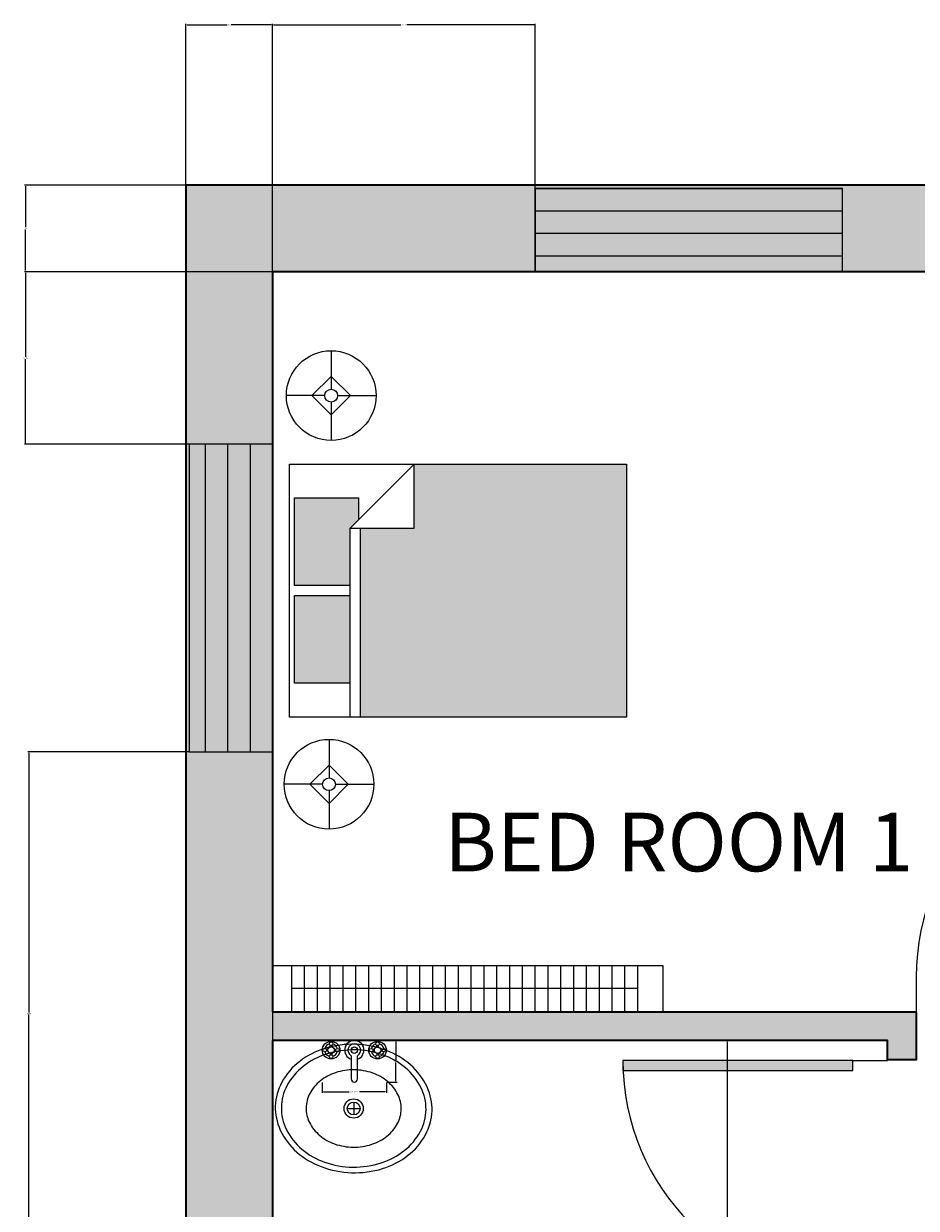
# Model space of a CAD drawing. Units: inches. Extents: x 1434 to 1845, y 1483 to 2014.
# Tile 9 of 11: x 1434 to 1573, y 1829 to 2014. Entities that reach past the tile are written whole.
import ezdxf

# ---------------------------------------------------------------- set-up
doc = ezdxf.new("R2010")
doc.units = ezdxf.units.IN
for name, color, linetype, lineweight in [('A-ANNO-DIMS', 2, 'Continuous', 18), ('A-AREA-IDEN', 7, 'Continuous', 25), ('A-DOOR', 3, 'Continuous', 25), ('A-FLOR-FIXT', 8, 'Continuous', 18), ('A-FLOR-FIXT-PATT', 8, 'Continuous', 13), ('A-FURN', 9, 'Continuous', 18), ('A-FURN-PATT', 9, 'Continuous', 13), ('A-GLAZ', 4, 'Continuous', 18), ('A-GLAZ-PATT', 9, 'Continuous', 13), ('A-WALL', 7, 'Continuous', 35), ('A-WALL-PATT', 8, 'Continuous', 13), ('E-LITE', 2, 'Continuous', 18)]:
    doc.layers.add(name, color=color, linetype=linetype, lineweight=lineweight)
doc.layers.add('A-DOOR-PATT', color=39, linetype='Continuous', lineweight=13, true_color=0x58382b)
doc.styles.get("Standard").update_dxf_attribs({"font": 'arial.ttf'})
doc.dimstyles.get("Standard").update_dxf_attribs({"dimtxt": 0.18, "dimasz": 0.18, "dimexe": 0.18, "dimexo": 0.0625, "dimgap": 0.09, "dimtad": 0, "dimtih": 1, "dimtoh": 1, "dimdec": 4, "dimzin": 0, "dimdsep": 46, "dimtxsty": 'Standard', "dimcen": 0.09, "dimadec": 0, "dimazin": 0, "dimtfac": 1, "dimtdec": 4, "dimtofl": 0, "dimtmove": 0, "dimatfit": 3, "dimfxl": 1, "dimtolj": 1, "dimtzin": 0, "dimarcsym": 0})

# ---------------------------------------------------------------- blocks, each defined once
blk = doc.blocks.new('*U2')
for p, q in [((0, 0), (0, -6)), ((-40, 0), (-40, -6))]:
    blk.add_line(p, q)
blk.add_lwpolyline([(0, 0), (0, 40), (-1.75, 40), (-1.75, 0)], close=True)
blk.add_arc((0, 0), 40, 90, 180)
blk = doc.blocks.new('Bed - Queen')
for p, q in [((0, -80.00003), (0, 0)), ((0, 0), (59.99999, 0)), ((59.99999, 0), (59.99999, -80.00003)), ((7.99999, -1.2), (28.79998, -1.2)), ((7.99999, -14.4), (7.99999, -1.2)), ((28.79998, -1.2), (28.79998, -14.4)), ((31.19999, -1.2), (51.99999, -1.2)), ((31.19999, -14.4), (31.19999, -1.2)), ((51.99999, -1.2), (51.99999, -16.4)), ((0, -14.4), (44.8, -14.4)), ((44.8, -16.8), (0, -16.8)), ((59.99999, -29.6), (44.8, -14.4)), ((44.8, -14.4), (44.8, -29.6)), ((51.99999, -16.4), (46.79936, -16.4)), ((44.8, -29.6), (59.99999, -29.6)), ((59.99999, -80.00003), (0, -80.00003))]:
    blk.add_line(p, q)
blk = doc.blocks.new('Lamp - Table')
for p, q in [((0, 7), (0, 1)), ((0, 3), (-3, 0)), ((3, 0), (0, 3)), ((-1, 0), (-7, 0)), ((-3, 0), (0, -3)), ((0, -3), (3, 0)), ((1, 0), (7, 0)), ((0, -1), (0, -7))]:
    blk.add_line(p, q)
for radius in [7, 1]:
    blk.add_circle((0, 0), radius)
blk = doc.blocks.new('Sink - Oval top')
for p, q in [((-1, 0), (1, 0)), ((0, 1), (0, -1))]:
    blk.add_line(p, q)
for points in [[(-12.23, 0.39, 0.117634), (-11.46, -3.36, 0.104469), (-8.88, -6.8, 0.090016), (-5.08, -9.07, 0.08192), (-0.32, -10.02, 0.08192), (4.49, -9.38, 0.090016), (8.42, -7.36, 0.104469), (11.22, -4.09, 0.117634), (12.23, -0.39, 0.117634), (11.46, 3.36, 0.104469), (8.88, 6.8, 0.090016), (5.08, 9.07, 0.08192), (0.32, 10.02, 0.08192), (-4.49, 9.38, 0.090016), (-8.42, 7.36, 0.104469), (-11.22, 4.09, 0.117634)], [(-11.29, 0.16, 0.118622), (-10.52, -3.25, 0.104678), (-8.07, -6.36, 0.089562), (-4.54, -8.37, 0.081185), (-0.13, -9.15, 0.081185), (4.3, -8.49, 0.089562), (7.89, -6.58, 0.104678), (10.42, -3.55, 0.118622), (11.29, -0.16, 0.118622), (10.52, 3.25, 0.104678), (8.07, 6.36, 0.089562), (4.54, 8.37, 0.081185), (0.13, 9.15, 0.081185), (-4.3, 8.49, 0.089562), (-7.89, 6.58, 0.104678), (-10.42, 3.55, 0.118622)], [(-7.42, 0.08, 0.118283), (-6.91, -2.17, 0.104607), (-5.29, -4.21, 0.089718), (-2.97, -5.53, 0.081436), (-0.07, -6.04, 0.081436), (2.84, -5.59, 0.089718), (5.2, -4.33, 0.104607), (6.86, -2.32, 0.118283), (7.42, -0.08, 0.118283), (6.91, 2.17, 0.104607), (5.29, 4.21, 0.089718), (2.97, 5.53, 0.081436), (0.07, 6.04, 0.081436), (-2.84, 5.59, 0.089718), (-5.2, 4.33, 0.104607), (-6.86, 2.32, 0.118283)]]:
    blk.add_lwpolyline(points, format="xyb", close=True)
for radius in [1.5, 1]:
    blk.add_circle((0, 0), radius)
blk = doc.blocks.new('Faucet - Bathroom top')
for p, q in [((-4.107, 0.125), (-4.375, 0.125)), ((-3.75, 0.4788), (-3.75, 0.75)), ((-3.5, 0.482), (-3.5, 0.75)), ((-3.1461, 0.125), (-2.875, 0.125)), ((3.143, 0.125), (2.875, 0.125)), ((3.5, 0.4788), (3.5, 0.75)), ((3.75, 0.482), (3.75, 0.75)), ((4.1039, 0.125), (4.375, 0.125)), ((-4.1039, -0.125), (-4.375, -0.125)), ((-3.75, -0.4821), (-3.75, -0.75)), ((-3.5, -0.4789), (-3.5, -0.75)), ((-3.143, -0.125), (-2.875, -0.125)), ((-0.5, -0.8639), (-0.5, -4.5)), ((0.5, -4.5), (0.5, -0.8631)), ((3.1461, -0.125), (2.875, -0.125)), ((3.5, -0.4821), (3.5, -0.75)), ((3.75, -0.4789), (3.75, -0.75)), ((4.107, -0.125), (4.375, -0.125))]:
    blk.add_line(p, q)
for centre, radius in [((-3.625, 0), 1.375), ((-4.625, 0), 0.2795), ((-3.625, 0), 0.5), ((-3.625, 1), 0.2795), ((-2.625, 0), 0.2795), ((0, 0), 0.5), ((3.625, 0), 1.375), ((2.625, 0), 0.2795), ((3.625, 0), 0.5), ((3.625, 1), 0.2795), ((4.625, 0), 0.2795), ((-3.625, -1), 0.2795), ((3.625, -1), 0.2795)]:
    blk.add_circle(centre, radius)
for centre, radius, start, end in [((-3.625, 0), 1, 105.2407, 164.2093), ((-3.625, 0), 1, 16.44125, 74.07887), ((0, 0), 1.5, 289.6514, 250.3603), ((0, 0), 1, 300.3431, 239.7554), ((3.625, 0), 1, 106.12, 164.0884), ((3.625, 0), 1, 16.23422, 73.90469), ((-3.625, 0), 1, 196.2342, 253.9047), ((-3.625, 0), 1, 286.12, 344.0884), ((3.625, 0), 1, 196.4413, 254.0789), ((3.625, 0), 1, 285.2407, 344.2093), ((0, -4.5), 0.5, 180, 0)]:
    blk.add_arc(centre, radius, start, end)
blk = doc.blocks.new('WIN-48IN-13IN')
for p, q in [((13, 48), (0, 48)), ((0, 48), (0, 12)), ((2.5, 48), (2.5, 0)), ((6, 48), (6, 0)), ((9.5, 48), (9.5, 0)), ((0, 12), (0, 0)), ((0, 0), (13, 0))]:
    blk.add_line(p, q)
blk.add_lwpolyline([(13, 48), (13, 0)], close=True)
blk = doc.blocks.new('*D34')
at = {"layer": 'A-ANNO-DIMS', "color": 0, "lineweight": -2, "transparency": 16777216}
for p, q in [((1480.75, 1848.31), (1480.75, 1846.69)), ((1480.93, 1846.87), (1484.94, 1846.87)), ((1490.57, 1846.87), (1486.56, 1846.87)), ((1490.75, 1848.31), (1490.75, 1846.69))]:
    blk.add_line(p, q, dxfattribs=at)
at = {"layer": 'A-ANNO-DIMS', "color": 0, "transparency": 16777216}
for points in [[(1480.93, 1846.9), (1480.93, 1846.84), (1480.75, 1846.87)], [(1490.57, 1846.9), (1490.57, 1846.84), (1490.75, 1846.87)]]:
    blk.add_solid(points, dxfattribs=at)
at = {"layer": 'Defpoints', "color": 0, "transparency": 16777216}
for p in [(1480.75, 1848.37), (1490.75, 1848.37), (1490.75, 1846.87)]:
    blk.add_point(p, dxfattribs=at)
at = {"layer": 'A-ANNO-DIMS', "color": 0, "transparency": 16777216, "insert": (1485.75, 1846.87), "char_height": 0.18, "attachment_point": 5}
blk.add_mtext('\\A1;TAP 10 TYP.', dxfattribs=at)
blk = doc.blocks.new('*D35')
at = {"layer": 'A-ANNO-DIMS', "color": 0, "lineweight": -2, "transparency": 16777216}
for p, q in [((1490.81, 1854.87), (1492.43, 1854.87)), ((1492.25, 1854.69), (1492.25, 1851.8)), ((1492.25, 1848.55), (1492.25, 1851.44)), ((1490.81, 1848.37), (1492.43, 1848.37))]:
    blk.add_line(p, q, dxfattribs=at)
at = {"layer": 'A-ANNO-DIMS', "color": 0, "transparency": 16777216}
for points in [[(1492.22, 1854.69), (1492.28, 1854.69), (1492.25, 1854.87)], [(1492.22, 1848.55), (1492.28, 1848.55), (1492.25, 1848.37)]]:
    blk.add_solid(points, dxfattribs=at)
at = {"layer": 'Defpoints', "color": 0, "transparency": 16777216}
for p in [(1490.75, 1854.87), (1492.25, 1854.87), (1490.75, 1848.37)]:
    blk.add_point(p, dxfattribs=at)
at = {"layer": 'A-ANNO-DIMS', "color": 0, "transparency": 16777216, "insert": (1492.25, 1851.62), "char_height": 0.18, "attachment_point": 5}
blk.add_mtext('\\A1;7 TYP.', dxfattribs=at)
blk = doc.blocks.new('*D56')
at = {"layer": 'A-ANNO-DIMS', "color": 0, "lineweight": -2, "transparency": 16777216}
for p, q in [((1472.97, 1974.79), (1472.97, 1483.15)), ((1612.47, 1974.79), (1612.47, 1483.15)), ((1473.15, 1483.33), (1542.34, 1483.33)), ((1612.29, 1483.33), (1543.11, 1483.33))]:
    blk.add_line(p, q, dxfattribs=at)
at = {"layer": 'A-ANNO-DIMS', "color": 0, "transparency": 16777216}
for points in [[(1473.15, 1483.36), (1473.15, 1483.3), (1472.97, 1483.33)], [(1612.29, 1483.36), (1612.29, 1483.3), (1612.47, 1483.33)]]:
    blk.add_solid(points, dxfattribs=at)
at = {"layer": 'Defpoints', "color": 0, "transparency": 16777216}
for p in [(1472.97, 1974.86), (1612.47, 1974.86), (1612.47, 1483.33)]:
    blk.add_point(p, dxfattribs=at)
at = {"layer": 'A-ANNO-DIMS', "color": 0, "transparency": 16777216, "insert": (1542.72, 1483.33), "char_height": 0.18, "attachment_point": 5}
blk.add_mtext('\\A1;139.5', dxfattribs=at)
blk = doc.blocks.new('*D63')
at = {"layer": 'A-ANNO-DIMS', "color": 0, "lineweight": -2, "transparency": 16777216}
for p, q in [((1568.91, 1854.86), (1543.77, 1854.86)), ((1543.95, 1854.68), (1543.95, 1795.04)), ((1543.95, 1735.04), (1543.95, 1794.67)), ((1568.91, 1734.86), (1543.77, 1734.86))]:
    blk.add_line(p, q, dxfattribs=at)
at = {"layer": 'A-ANNO-DIMS', "color": 0, "transparency": 16777216}
for points in [[(1543.92, 1854.68), (1543.98, 1854.68), (1543.95, 1854.86)], [(1543.92, 1735.04), (1543.98, 1735.04), (1543.95, 1734.86)]]:
    blk.add_solid(points, dxfattribs=at)
at = {"layer": 'Defpoints', "color": 0, "transparency": 16777216}
for p in [(1543.95, 1854.86), (1568.97, 1854.86), (1568.97, 1734.86)]:
    blk.add_point(p, dxfattribs=at)
at = {"layer": 'A-ANNO-DIMS', "color": 0, "transparency": 16777216, "insert": (1543.95, 1794.86), "char_height": 0.18, "attachment_point": 5}
blk.add_mtext('\\A1;120', dxfattribs=at)
blk = doc.blocks.new('*D74')
at = {"layer": 'A-ANNO-DIMS', "color": 0, "lineweight": -2, "transparency": 16777216}
for p, q in [((1472.97, 1974.92), (1472.97, 2013.56)), ((1473.15, 2013.38), (1493.01, 2013.38)), ((1513.8, 2013.38), (1493.94, 2013.38)), ((1513.98, 1974.92), (1513.98, 2013.56))]:
    blk.add_line(p, q, dxfattribs=at)
at = {"layer": 'A-ANNO-DIMS', "color": 0, "transparency": 16777216}
for points in [[(1473.15, 2013.41), (1473.15, 2013.35), (1472.97, 2013.38)], [(1513.8, 2013.41), (1513.8, 2013.35), (1513.98, 2013.38)]]:
    blk.add_solid(points, dxfattribs=at)
at = {"layer": 'Defpoints', "color": 0, "transparency": 16777216}
for p in [(1513.98, 2013.38), (1472.97, 1974.86), (1513.98, 1974.86)]:
    blk.add_point(p, dxfattribs=at)
at = {"layer": 'A-ANNO-DIMS', "color": 0, "transparency": 16777216, "insert": (1493.48, 2013.38), "char_height": 0.18, "attachment_point": 5}
blk.add_mtext('\\A1;41.004', dxfattribs=at)
blk = doc.blocks.new('*D76')
at = {"layer": 'A-ANNO-DIMS', "color": 0, "lineweight": -2, "transparency": 16777216}
for p, q in [((1472.91, 1974.86), (1434.27, 1974.86)), ((1434.45, 1974.68), (1434.45, 1961.58)), ((1434.45, 1948.12), (1434.45, 1961.21)), ((1472.91, 1947.94), (1434.27, 1947.94))]:
    blk.add_line(p, q, dxfattribs=at)
at = {"layer": 'A-ANNO-DIMS', "color": 0, "transparency": 16777216}
for points in [[(1434.42, 1974.68), (1434.48, 1974.68), (1434.45, 1974.86)], [(1434.42, 1948.12), (1434.48, 1948.12), (1434.45, 1947.94)]]:
    blk.add_solid(points, dxfattribs=at)
at = {"layer": 'Defpoints', "color": 0, "transparency": 16777216}
for p in [(1434.45, 1974.86), (1472.97, 1974.86), (1472.97, 1947.94)]:
    blk.add_point(p, dxfattribs=at)
at = {"layer": 'A-ANNO-DIMS', "color": 0, "transparency": 16777216, "insert": (1434.45, 1961.4), "char_height": 0.18, "attachment_point": 5}
blk.add_mtext('\\A1;26.92', dxfattribs=at)
blk = doc.blocks.new('*D77')
at = {"layer": 'A-ANNO-DIMS', "color": 0, "lineweight": -2, "transparency": 16777216}
for p, q in [((1459.91, 1899.94), (1434.77, 1899.94)), ((1434.95, 1899.76), (1434.95, 1859.25)), ((1434.95, 1818.38), (1434.95, 1858.88)), ((1459.91, 1818.2), (1434.77, 1818.2))]:
    blk.add_line(p, q, dxfattribs=at)
at = {"layer": 'A-ANNO-DIMS', "color": 0, "transparency": 16777216}
for points in [[(1434.92, 1899.76), (1434.98, 1899.76), (1434.95, 1899.94)], [(1434.92, 1818.38), (1434.98, 1818.38), (1434.95, 1818.2)]]:
    blk.add_solid(points, dxfattribs=at)
at = {"layer": 'Defpoints', "color": 0, "transparency": 16777216}
for p in [(1434.95, 1899.94), (1459.97, 1899.94), (1459.97, 1818.2)]:
    blk.add_point(p, dxfattribs=at)
at = {"layer": 'A-ANNO-DIMS', "color": 0, "transparency": 16777216, "insert": (1434.95, 1859.07), "char_height": 0.18, "attachment_point": 5}
blk.add_mtext('\\A1;81.74', dxfattribs=at)
blk = doc.blocks.new('*D87')
at = {"layer": 'A-ANNO-DIMS', "color": 0, "lineweight": -2, "transparency": 16777216}
for p, q in [((1459.41, 1988.36), (1434.27, 1988.36)), ((1434.45, 1988.18), (1434.45, 1981.79)), ((1434.45, 1975.04), (1434.45, 1981.42)), ((1472.91, 1974.86), (1434.27, 1974.86))]:
    blk.add_line(p, q, dxfattribs=at)
at = {"layer": 'A-ANNO-DIMS', "color": 0, "transparency": 16777216}
for points in [[(1434.42, 1988.18), (1434.48, 1988.18), (1434.45, 1988.36)], [(1434.42, 1975.04), (1434.48, 1975.04), (1434.45, 1974.86)]]:
    blk.add_solid(points, dxfattribs=at)
at = {"layer": 'Defpoints', "color": 0, "transparency": 16777216}
for p in [(1459.47, 1988.36), (1434.45, 1974.86), (1472.97, 1974.86)]:
    blk.add_point(p, dxfattribs=at)
at = {"layer": 'A-ANNO-DIMS', "color": 0, "transparency": 16777216, "insert": (1434.45, 1981.61), "char_height": 0.18, "attachment_point": 5}
blk.add_mtext('\\A1;13.5', dxfattribs=at)
blk = doc.blocks.new('*D88')
at = {"layer": 'A-ANNO-DIMS', "color": 0, "lineweight": -2, "transparency": 16777216}
for p, q in [((1459.47, 1988.42), (1459.47, 2013.56)), ((1459.65, 2013.38), (1465.91, 2013.38)), ((1472.79, 2013.38), (1466.54, 2013.38)), ((1472.97, 1974.92), (1472.97, 2013.56))]:
    blk.add_line(p, q, dxfattribs=at)
at = {"layer": 'A-ANNO-DIMS', "color": 0, "transparency": 16777216}
for points in [[(1459.65, 2013.41), (1459.65, 2013.35), (1459.47, 2013.38)], [(1472.79, 2013.41), (1472.79, 2013.35), (1472.97, 2013.38)]]:
    blk.add_solid(points, dxfattribs=at)
at = {"layer": 'Defpoints', "color": 0, "transparency": 16777216}
for p in [(1472.97, 2013.38), (1459.47, 1988.36), (1472.97, 1974.86)]:
    blk.add_point(p, dxfattribs=at)
at = {"layer": 'A-ANNO-DIMS', "color": 0, "transparency": 16777216, "insert": (1466.22, 2013.38), "char_height": 0.18, "attachment_point": 5}
blk.add_mtext('\\A1;13.5', dxfattribs=at)

msp = doc.modelspace()

# ---------------------------------------------------------------- hatches: boundary and pattern name
at = {"layer": 'A-DOOR-PATT'}
h = msp.add_hatch(color=256, dxfattribs=at)
h.dxf.hatch_style = 1
h.paths.add_polyline_path([(1611.5864, 1583.2737), (1575.6681, 1583.2737, 0.01094143), (1575.7025, 1581.7022), (1611.5864, 1581.7022)])
h.paths.add_polyline_path([(1621.4742, 1547.3553), (1616.9742, 1547.3553), (1616.9742, 1544.3553), (1621.4742, 1544.3553)])
h.paths.add_polyline_path([(1635.0456, 1558.627, 0.01094143), (1633.4742, 1558.6614), (1633.4742, 1522.7431), (1635.0456, 1522.7431)])
h.paths.add_polyline_path([(1633.4742, 1517.3553), (1630.4742, 1517.3553), (1630.4742, 1508.3553), (1633.4742, 1508.3553)])
h.paths.add_polyline_path([(1672.8212, 1517.3553), (1669.8212, 1517.3553), (1669.8212, 1508.3553), (1672.8212, 1508.3553)])
h.paths.add_polyline_path([(1613.8925, 1724.9676), (1612.3211, 1724.9676), (1612.3211, 1689.0836, 0.01094143), (1613.8925, 1689.0492)])
h.paths.add_polyline_path([(1789.3925, 1684.9726), (1753.4742, 1684.9726), (1753.4742, 1683.4011), (1789.3925, 1683.4011)])
h.paths.add_polyline_path([(1792.4742, 1679.5848), (1789.4742, 1679.5848), (1789.4742, 1675.0848), (1792.4742, 1675.0848)])
h.paths.add_polyline_path([(1563.5864, 1851.7737), (1527.6681, 1851.7737, 0.01094143), (1527.7025, 1850.2022), (1563.5864, 1850.2022)])
h.paths.add_polyline_path([(1609.3925, 1900.6614, 0.01094143), (1607.8211, 1900.627), (1607.8211, 1864.7431), (1609.3925, 1864.7431)])
h.paths.add_polyline_path([(1675.5456, 1900.627, 0.01094143), (1673.9742, 1900.6614), (1673.9742, 1864.7431), (1675.5456, 1864.7431)])
h.paths.add_polyline_path([(1751.2803, 1851.8553), (1715.3619, 1851.8553), (1715.3619, 1850.2839), (1751.2459, 1850.2839, 0.01094143)])
at = {"layer": 'A-FLOR-FIXT-PATT'}
h = msp.add_hatch(dxfattribs=at)
h.set_pattern_fill('ANSI31', color=256, scale=0.629921, angle=45, style=0)
h.paths.add_polyline_path([(1474.8993, 1859.3553), (1530.8993, 1859.3553), (1530.8993, 1866.5838), (1474.8993, 1866.5838)])
at = {"layer": 'A-FURN-PATT'}
h = msp.add_hatch(color=256, dxfattribs=at)
h.dxf.hatch_style = 1
h.paths.add_polyline_path([(1528.2614, 1944.8381), (1495.0961, 1944.8381), (1495.0961, 1934.8359), (1486.6731, 1934.8359), (1486.6731, 1905.3556), (1528.2614, 1905.3556)])
h.paths.add_polyline_path([(1796.7541, 1950.9116), (1755.1658, 1950.9116), (1755.1658, 1911.4291), (1788.3311, 1911.4291), (1788.3311, 1921.4313), (1796.7541, 1921.4313)])
h.paths.add_polyline_path([(1529.423, 1679.282), (1496.2577, 1679.282), (1496.2577, 1669.2798), (1487.8347, 1669.2798), (1487.8347, 1639.7996), (1529.423, 1639.7996)])
h.paths.add_polyline_path([(1486.2554, 1669.2798), (1487.5715, 1670.5959), (1487.5715, 1674.0177), (1477.5693, 1674.0177), (1477.5693, 1660.3304), (1486.2554, 1660.3304)])
h.paths.add_polyline_path([(1486.2554, 1658.7511), (1477.5693, 1658.7511), (1477.5693, 1645.0639), (1486.2554, 1645.0639)])
h.paths.add_polyline_path([(1807.0195, 1930.3807), (1798.3334, 1930.3807), (1798.3334, 1921.4313), (1797.0173, 1920.1152), (1797.0173, 1916.6934), (1807.0195, 1916.6934)])
h.paths.add_polyline_path([(1807.0195, 1945.6472), (1798.3334, 1945.6472), (1798.3334, 1931.96), (1807.0195, 1931.96)])
h.paths.add_polyline_path([(1485.0938, 1934.8359), (1486.4099, 1936.152), (1486.4099, 1939.5738), (1476.4077, 1939.5738), (1476.4077, 1925.8865), (1485.0938, 1925.8865)])
h.paths.add_polyline_path([(1485.0938, 1924.3072), (1476.4077, 1924.3072), (1476.4077, 1910.62), (1485.0938, 1910.62)])
at = {"layer": 'A-GLAZ-PATT'}
h = msp.add_hatch(color=256, dxfattribs=at)
h.dxf.hatch_style = 1
h.set_gradient(color1=(0, 0, 255), color2=(255, 255, 0), name='INVSPHERICAL')
h.paths.add_polyline_path([(1561.9785, 1987.8553), (1513.9785, 1987.8553), (1513.9785, 1984.3553), (1561.9785, 1984.3553)])
h.paths.add_polyline_path([(1561.9785, 1984.3553), (1513.9785, 1984.3553), (1513.9785, 1980.8553), (1561.9785, 1980.8553)])
h.paths.add_polyline_path([(1561.9785, 1980.8553), (1513.9785, 1980.8553), (1513.9785, 1977.3553), (1561.9785, 1977.3553)])
h.paths.add_polyline_path([(1561.9785, 1977.3553), (1513.9785, 1977.3553), (1513.9785, 1974.8553), (1549.9785, 1974.8553), (1561.9785, 1974.8553)])
h = msp.add_hatch(color=256, dxfattribs=at)
h.dxf.hatch_style = 1
h.set_gradient(color1=(0, 0, 255), color2=(255, 255, 0), name='INVCYLINDER')
h.paths.add_polyline_path([(1462.4742, 1947.9369), (1459.9742, 1947.9369), (1459.9742, 1911.9369), (1459.9742, 1899.9369), (1462.4742, 1899.9369)])
h.paths.add_polyline_path([(1465.9742, 1947.9369), (1462.4742, 1947.9369), (1462.4742, 1899.9369), (1465.9742, 1899.9369)])
h.paths.add_polyline_path([(1472.9742, 1947.9369), (1469.4742, 1947.9369), (1469.4742, 1899.9369), (1472.9742, 1899.9369)])
h.paths.add_polyline_path([(1469.4742, 1947.9369), (1465.9742, 1947.9369), (1465.9742, 1899.9369), (1469.4742, 1899.9369)])
at = {"layer": 'A-WALL-PATT'}
h = msp.add_hatch(color=256, dxfattribs=at)
h.dxf.hatch_style = 1
h.paths.add_polyline_path([(1472.9742, 1730.3553), (1577.9742, 1730.3553), (1577.9742, 1734.8553), (1573.4742, 1734.8553), (1573.4742, 1815.8553), (1568.9742, 1815.8553), (1568.9742, 1734.8553), (1472.9742, 1734.8553), (1472.9742, 1770.1951), (1459.9742, 1770.1951), (1459.9742, 1782.1951), (1459.9742, 1818.1951), (1472.9742, 1818.1951), (1472.9742, 1854.8553), (1568.9742, 1854.8553), (1568.9742, 1851.8553), (1573.4742, 1851.8553), (1573.4742, 1854.8553), (1573.4742, 1859.3553), (1472.9742, 1859.3553), (1472.9742, 1899.9369), (1459.9742, 1899.9369), (1459.9742, 1911.9369), (1459.9742, 1947.9369), (1472.9742, 1947.9369), (1472.9742, 1974.8553), (1513.9785, 1974.8553), (1513.9785, 1987.8553), (1561.9785, 1987.8553), (1561.9785, 1974.8553), (1612.4742, 1974.8553), (1612.4742, 1859.3553), (1609.4742, 1859.3553), (1609.4742, 1854.8553), (1616.9742, 1854.8553), (1616.9742, 1910.3553), (1625.153, 1910.3553), (1625.153, 1914.8553), (1616.9742, 1914.8553), (1616.9742, 1988.3553), (1459.4742, 1988.3553), (1459.4742, 1508.3553), (1630.4742, 1508.3553), (1630.4742, 1517.3553), (1472.9742, 1517.3553), (1472.9742, 1586.3553), (1616.9742, 1586.3553), (1616.9742, 1583.3553), (1621.4742, 1583.3553), (1621.4742, 1586.3553), (1621.4742, 1734.8553), (1616.9742, 1734.8553), (1613.9742, 1734.8553), (1613.9742, 1730.3553), (1616.9742, 1730.3553), (1616.9742, 1590.8553), (1472.9742, 1590.8553), (1472.9742, 1635.7299), (1459.9742, 1635.7299), (1459.9742, 1647.7299), (1459.9742, 1683.7299), (1472.9742, 1683.7299)])
h.paths.add_polyline_path([(1819.4742, 1773.1667), (1810.4742, 1773.1667), (1810.4742, 1734.8553), (1714.4742, 1734.8553), (1714.4742, 1815.8553), (1709.9742, 1815.8553), (1709.9742, 1730.3553), (1745.9742, 1730.3553), (1745.9742, 1675.0848), (1753.4742, 1675.0848), (1753.4742, 1679.5848), (1750.4742, 1679.5848), (1750.4742, 1730.3553), (1810.4742, 1730.3553), (1810.4742, 1679.5848), (1792.4742, 1679.5848), (1792.4742, 1675.0848), (1810.4742, 1675.0848), (1810.4742, 1517.3553), (1775.1129, 1517.3553), (1775.1129, 1508.3553), (1819.4742, 1508.3553)])
h.paths.add_polyline_path([(1739.1129, 1517.3553), (1694.9742, 1517.3553), (1694.9742, 1730.3553), (1690.4742, 1730.3553), (1690.4742, 1517.3553), (1678.4742, 1517.3553), (1675.4742, 1517.3553), (1672.8212, 1517.3553), (1672.8212, 1508.3553), (1678.4742, 1508.3553), (1739.1129, 1508.3553)])
h.paths.add_polyline_path([(1735.6549, 1987.8553), (1783.6549, 1987.8553), (1783.6549, 1974.8553), (1810.4742, 1974.8553), (1810.4742, 1859.3553), (1709.9742, 1859.3553), (1709.9742, 1854.8553), (1709.9742, 1851.8553), (1714.4742, 1851.8553), (1714.4742, 1854.8553), (1810.4742, 1854.8553), (1810.4742, 1809.1667), (1819.4742, 1809.1667), (1819.4742, 1988.3553), (1666.4742, 1988.3553), (1666.4742, 1914.8553), (1661.1087, 1914.8553), (1661.1087, 1910.3553), (1666.4742, 1910.3553), (1666.4742, 1854.8553), (1673.9742, 1854.8553), (1673.9742, 1859.3553), (1670.9742, 1859.3553), (1670.9742, 1974.8553), (1735.6549, 1974.8553)])

# ---------------------------------------------------------------- linework, layer by layer
at = {"layer": 'A-FLOR-FIXT'}
for p, q in [((1472.9742, 1866.5838), (1533.8993, 1866.5838)), ((1472.9742, 1859.3553), (1472.9742, 1866.5838)), ((1533.8993, 1866.5838), (1533.8993, 1859.3553)), ((1529.8993, 1862.9695), (1475.8993, 1862.9695)), ((1533.8993, 1859.3553), (1472.9742, 1859.3553))]:
    msp.add_line(p, q, dxfattribs=at)
at = {"layer": 'A-WALL'}
for p, q in [((1472.9742, 1974.8553), (1472.9742, 1859.3553)), ((1612.4742, 1974.8553), (1472.9742, 1974.8553)), ((1472.9742, 1854.8553), (1472.9742, 1734.8553))]:
    msp.add_line(p, q, dxfattribs=at)
for points in [[(1678.4742, 1508.3553), (1819.4742, 1508.3553), (1819.4742, 1988.3553), (1459.4742, 1988.3553), (1459.4742, 1508.3553), (1630.4742, 1508.3553)], [(1472.9742, 1859.3553), (1573.4742, 1859.3553), (1573.4742, 1854.8553), (1573.4742, 1851.8553), (1568.9742, 1851.8553), (1568.9742, 1854.8553), (1472.9742, 1854.8553)]]:
    msp.add_lwpolyline(points, dxfattribs=at)

# ---------------------------------------------------------------- block references
at = {"layer": 'A-DOOR', "xscale": 0.8979587755198419, "yscale": 0.8979587755198419, "zscale": 0.8979587755198419}
msp.add_blockref('*U2', (1609.3925, 1864.7431), dxfattribs=at)
at = {"layer": 'A-DOOR', "xscale": 0.8979587755198419, "yscale": 0.8979587755198419, "zscale": 0.8979587755198419, "rotation": 90}
msp.add_blockref('*U2', (1563.5864, 1851.7737), dxfattribs=at)
at = {"layer": 'A-FLOR-FIXT'}
for name, p in [('Sink - Oval top', (1485.6514, 1844.2664)), ('Faucet - Bathroom top', (1485.7516, 1853.3732))]:
    msp.add_blockref(name, p, dxfattribs=at)
at = {"layer": 'A-FURN', "xscale": 0.6580416786709006, "yscale": 0.6580416786709006, "zscale": 0.6580416786709006, "rotation": 90}
msp.add_blockref('Bed - Queen', (1475.618, 1905.3556), dxfattribs=at)
at = {"layer": 'A-GLAZ', "rotation": 90.00000000000058}
msp.add_blockref('WIN-48IN-13IN', (1561.9785, 1974.8553), dxfattribs=at)
at = {"layer": 'A-GLAZ'}
msp.add_blockref('WIN-48IN-13IN', (1459.9742, 1899.9369), dxfattribs=at)
at = {"layer": 'E-LITE'}
for p in [(1482.1407, 1955.5201), (1481.8035, 1894.8703)]:
    msp.add_blockref('Lamp - Table', p, dxfattribs=at)

# ---------------------------------------------------------------- texts
at = {"layer": 'A-AREA-IDEN'}
msp.add_text('BED ROOM 1', height=9.14668, dxfattribs=at).set_placement((1499.7903, 1881.2726))

# ---------------------------------------------------------------- dimensions: what is measured, and where the dimension line sits
at = {"layer": 'A-ANNO-DIMS'}
for base, p1, p2, override, picture, middle in [((1472.9742, 2013.3803), (1459.4742, 1988.3553), (1472.9742, 1974.8553), {"dimdec": 1, "dimlfac": 1, "dimrnd": 0, "dimzin": 0, "dimdsep": 46, "dimlunit": 2}, '*D88', (1466.2242, 2013.3803)), ((1513.9785, 2013.3803), (1472.9742, 1974.8553), (1513.9785, 1974.8553), {"dimdec": 3, "dimlfac": 1, "dimrnd": 0, "dimzin": 0, "dimdsep": 46, "dimlunit": 2}, '*D74', (1493.4764, 2013.3803)), ((1612.4742, 1483.3303), (1472.9742, 1974.8553), (1612.4742, 1974.8553), {"dimdec": 1, "dimlfac": 1, "dimrnd": 0, "dimzin": 0, "dimdsep": 46, "dimlunit": 2}, '*D56', (1542.7242, 1483.3303))]:
    dim = msp.add_linear_dim(base=base, p1=p1, p2=p2, dimstyle='Standard', override=override, dxfattribs=at)
    dim.commit()
    dim.dimension.update_dxf_attribs({"geometry": picture, "text_midpoint": middle})
for base, p1, p2, override, picture, middle in [((1434.4492, 1974.8553), (1459.4742, 1988.3553), (1472.9742, 1974.8553), {"dimdec": 1, "dimlfac": 1, "dimrnd": 0, "dimzin": 0, "dimdsep": 46, "dimlunit": 2}, '*D87', (1434.4492, 1981.6053)), ((1434.4492, 1974.8553), (1472.9742, 1947.9369), (1472.9742, 1974.8553), {"dimdec": 2, "dimlfac": 1, "dimrnd": 0, "dimzin": 0, "dimdsep": 46, "dimlunit": 2}, '*D76', (1434.4492, 1961.3961)), ((1434.9492, 1899.9369), (1459.9742, 1818.1951), (1459.9742, 1899.9369), {"dimdec": 2, "dimlfac": 1, "dimrnd": 0, "dimzin": 0, "dimdsep": 46, "dimlunit": 2}, '*D77', (1434.9492, 1859.066)), ((1543.9492, 1854.8553), (1568.9742, 1734.8553), (1568.9742, 1854.8553), {"dimdec": 0, "dimlfac": 1, "dimrnd": 0, "dimzin": 0, "dimdsep": 46, "dimlunit": 2}, '*D63', (1543.9492, 1794.8553))]:
    dim = msp.add_linear_dim(base=base, p1=p1, p2=p2, angle=90, dimstyle='Standard', override=override, dxfattribs=at)
    dim.commit()
    dim.dimension.update_dxf_attribs({"geometry": picture, "text_midpoint": middle})
dim = msp.add_linear_dim(base=(1492.2516, 1854.8733), p1=(1490.7516, 1848.3732), p2=(1490.7516, 1854.8733), angle=90, text='<> TYP.', dimstyle='Standard', override={"dimdec": 0, "dimlfac": 1, "dimrnd": 0, "dimzin": 0, "dimdsep": 46, "dimlunit": 2}, dxfattribs=at)
dim.commit()
dim.dimension.update_dxf_attribs({"geometry": '*D35', "text_midpoint": (1492.2516, 1851.6232)})
dim = msp.add_linear_dim(base=(1490.7516, 1846.8732), p1=(1480.7516, 1848.3732), p2=(1490.7516, 1848.3732), text='TAP <> TYP.', dimstyle='Standard', override={"dimdec": 0, "dimlfac": 1, "dimrnd": 0, "dimzin": 0, "dimdsep": 46, "dimlunit": 2}, dxfattribs=at)
dim.commit()
dim.dimension.update_dxf_attribs({"geometry": '*D34', "text_midpoint": (1485.7516, 1846.8732)})

doc.saveas('drawing.dxf')
